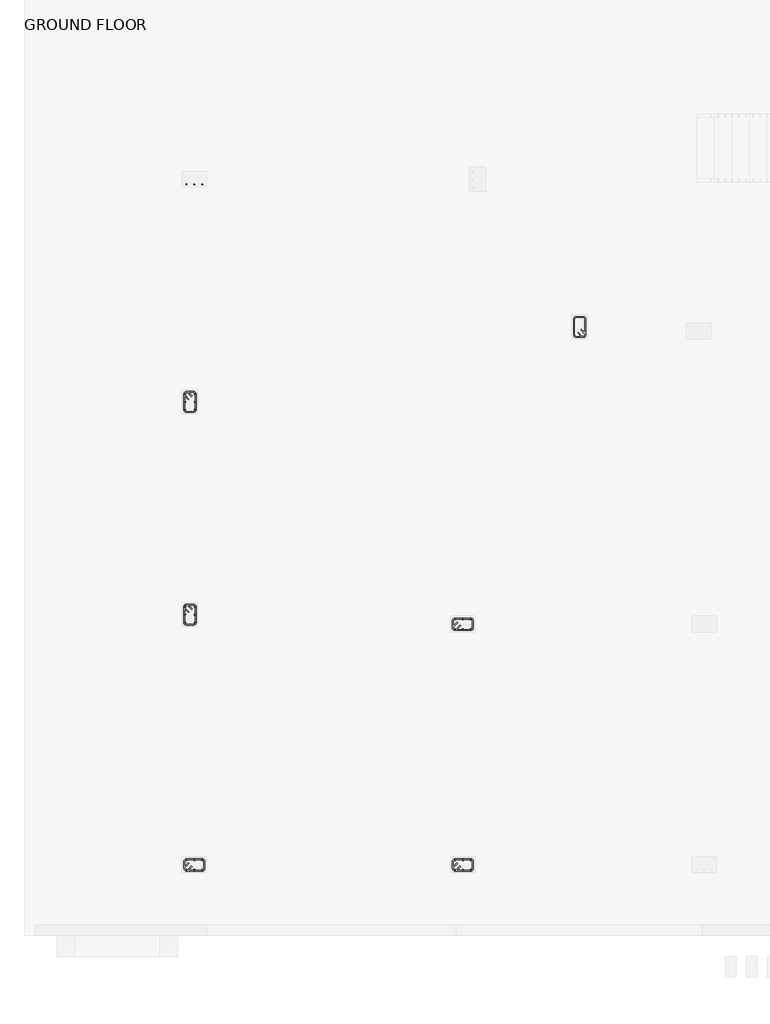
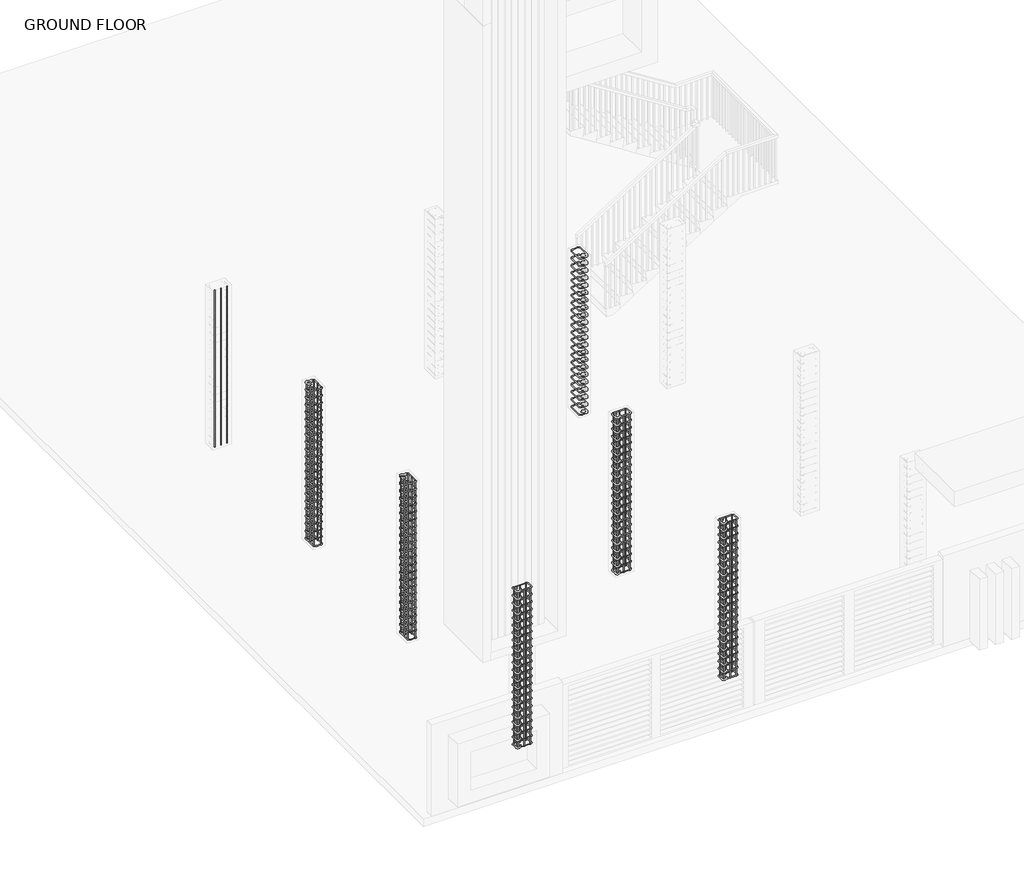
# One storey, part 3 of 7: 17 reinforcing bars.
"""IFC4 building model written with IfcOpenShell, lengths in millimetres."""

from ifc_helpers import new_model, si_unit, point, frame, origin, place, context, project, spatial, polyline, circle_curve, trimmed, segment, composite_curve, source, transform, mapped, element, save
from ifc_brep_helpers import swept_disk

model = new_model("IFC4")

# Units and contexts
model_context = context("Model", 3, world=origin())
ifc_project = project(units=[si_unit("LENGTHUNIT", "METRE", prefix="MILLI")], contexts=[model_context])

# Site, building, storey
site = spatial("IfcSite", under=ifc_project)
building = spatial("IfcBuilding", under=site)
storey = spatial("IfcBuildingStorey", under=building, Name="GROUND FLOOR", Elevation=0.0)

# Reinforcing bars
placement = place(None, origin())
reinforcing_bar_shape = source(origin(), model_context, "Body", "SolidModel", [
    swept_disk(composite_curve([segment(polyline([(-5960.0833787, -22.290066, 3175.0), (-5960.0833787, -22.290066, 25.4)]), True, "CONTINUOUS")], self_intersect=False), 6.35),
])
element("IfcReinforcingBar", 1, at=placement, inside=storey, context=model_context, shape_type="MappedRepresentation", body=[
    mapped(reinforcing_bar_shape, transform((0.0, 0.0, 0.0), x_axis=(1.0, 0.0, 0.0), y_axis=(0.0, 1.0, 0.0), z_axis=(0.0, 0.0, 1.0))),
    mapped(reinforcing_bar_shape, transform((-114.3, 0.0, 0.0), x_axis=(1.0, 0.0, 0.0), y_axis=(0.0, 1.0, 0.0), z_axis=(0.0, 0.0, 1.0))),
    mapped(reinforcing_bar_shape, transform((-228.6, 0.0, 0.0), x_axis=(1.0, 0.0, 0.0), y_axis=(0.0, 1.0, 0.0), z_axis=(0.0, 0.0, 1.0))),
])
reinforcing_bar_2_shape = source(origin(), model_context, "Body", "SolidModel", [
    swept_disk(composite_curve([segment(polyline([(-441.6142752, -2136.7078889, 3168.65), (-387.7327384, -2190.5894257, 3168.65)]), True, "CONTINUOUS"), segment(trimmed(circle_curve(frame((-410.1833787, -2213.040066, 3168.65), z_axis=(0.0, 0.0, -1.0), x_axis=(22.450640299999975, 22.450640300000032, 0.0)), 31.75), [point((-387.7327384, -2190.5894257, 3168.65))], [point((-410.1833787, -2244.790066, 3168.65))], True, "CARTESIAN"), True, "CONTINUOUS"), segment(polyline([(-410.1833787, -2244.790066, 3168.65), (-511.7833787, -2244.790066, 3168.65)]), True, "CONTINUOUS"), segment(trimmed(circle_curve(frame((-511.7833787, -2213.040066, 3168.65), z_axis=(0.0, 0.0, -1.0), x_axis=(0.0, -31.75, 0.0)), 31.75), [point((-511.7833787, -2244.790066, 3168.65))], [point((-543.5333787, -2213.040066, 3168.65))], True, "CARTESIAN"), True, "CONTINUOUS"), segment(polyline([(-543.5333787, -2213.040066, 3168.65), (-543.5333787, -1984.440066, 3168.65)]), True, "CONTINUOUS"), segment(trimmed(circle_curve(frame((-511.8768988, -1984.440066, 3171.0851138), z_axis=(0.07669649888473773, 0.0, -0.9970544855015816), x_axis=(-31.656479899999965, 0.0, -2.4351137999997263)), 31.75), [point((-543.5333787, -1984.440066, 3168.65))], [point((-511.8768988, -1952.690066, 3171.0851138))], True, "CARTESIAN"), True, "CONTINUOUS"), segment(polyline([(-511.8768988, -1952.690066, 3171.0851138), (-410.0898586, -1952.690066, 3178.9148862)]), True, "CONTINUOUS"), segment(trimmed(circle_curve(frame((-410.0898586, -1984.440066, 3178.9148862), z_axis=(0.07669649888473773, 0.0, -0.9970544855015816), x_axis=(0.0, 31.75, 0.0)), 31.75), [point((-410.0898586, -1952.690066, 3178.9148862))], [point((-378.4333787, -1984.440066, 3181.35))], True, "CARTESIAN"), True, "CONTINUOUS"), segment(polyline([(-378.4333787, -1984.440066, 3181.35), (-378.4333787, -2213.040066, 3181.35)]), True, "CONTINUOUS"), segment(trimmed(circle_curve(frame((-410.1833787, -2213.040066, 3181.35), z_axis=(0.0, 0.0, -1.0), x_axis=(31.75, 0.0, 0.0)), 31.75), [point((-378.4333787, -2213.040066, 3181.35))], [point((-432.634019, -2235.4907063, 3181.35))], True, "CARTESIAN"), True, "CONTINUOUS"), segment(polyline([(-432.634019, -2235.4907063, 3181.35), (-486.5155558, -2181.6091695, 3181.35)]), True, "CONTINUOUS")], self_intersect=False), 6.35),
])
element("IfcReinforcingBar", 2, at=placement, inside=storey, context=model_context, shape_type="MappedRepresentation", body=[
    mapped(reinforcing_bar_2_shape, transform((0.0, 0.0, 0.0), x_axis=(1.0, 0.0, 0.0), y_axis=(0.0, 1.0, 0.0), z_axis=(0.0, 0.0, 1.0))),
    mapped(reinforcing_bar_2_shape, transform((0.0, 0.0, -149.3761905), x_axis=(1.0, 0.0, 0.0), y_axis=(0.0, 1.0, 0.0), z_axis=(0.0, 0.0, 1.0))),
    mapped(reinforcing_bar_2_shape, transform((0.0, 0.0, -298.752381), x_axis=(1.0, 0.0, 0.0), y_axis=(0.0, 1.0, 0.0), z_axis=(0.0, 0.0, 1.0))),
    mapped(reinforcing_bar_2_shape, transform((0.0, 0.0, -448.1285714), x_axis=(1.0, 0.0, 0.0), y_axis=(0.0, 1.0, 0.0), z_axis=(0.0, 0.0, 1.0))),
    mapped(reinforcing_bar_2_shape, transform((0.0, 0.0, -597.5047619), x_axis=(1.0, 0.0, 0.0), y_axis=(0.0, 1.0, 0.0), z_axis=(0.0, 0.0, 1.0))),
    mapped(reinforcing_bar_2_shape, transform((0.0, 0.0, -746.8809524), x_axis=(1.0, 0.0, 0.0), y_axis=(0.0, 1.0, 0.0), z_axis=(0.0, 0.0, 1.0))),
    mapped(reinforcing_bar_2_shape, transform((0.0, 0.0, -896.2571429), x_axis=(1.0, 0.0, 0.0), y_axis=(0.0, 1.0, 0.0), z_axis=(0.0, 0.0, 1.0))),
    mapped(reinforcing_bar_2_shape, transform((0.0, 0.0, -1045.6333333), x_axis=(1.0, 0.0, 0.0), y_axis=(0.0, 1.0, 0.0), z_axis=(0.0, 0.0, 1.0))),
    mapped(reinforcing_bar_2_shape, transform((0.0, 0.0, -1195.0095238), x_axis=(1.0, 0.0, 0.0), y_axis=(0.0, 1.0, 0.0), z_axis=(0.0, 0.0, 1.0))),
    mapped(reinforcing_bar_2_shape, transform((0.0, 0.0, -1344.3857143), x_axis=(1.0, 0.0, 0.0), y_axis=(0.0, 1.0, 0.0), z_axis=(0.0, 0.0, 1.0))),
    mapped(reinforcing_bar_2_shape, transform((0.0, 0.0, -1493.7619048), x_axis=(1.0, 0.0, 0.0), y_axis=(0.0, 1.0, 0.0), z_axis=(0.0, 0.0, 1.0))),
    mapped(reinforcing_bar_2_shape, transform((0.0, 0.0, -1643.1380952), x_axis=(1.0, 0.0, 0.0), y_axis=(0.0, 1.0, 0.0), z_axis=(0.0, 0.0, 1.0))),
    mapped(reinforcing_bar_2_shape, transform((0.0, 0.0, -1792.5142857), x_axis=(1.0, 0.0, 0.0), y_axis=(0.0, 1.0, 0.0), z_axis=(0.0, 0.0, 1.0))),
    mapped(reinforcing_bar_2_shape, transform((0.0, 0.0, -1941.8904762), x_axis=(1.0, 0.0, 0.0), y_axis=(0.0, 1.0, 0.0), z_axis=(0.0, 0.0, 1.0))),
    mapped(reinforcing_bar_2_shape, transform((0.0, 0.0, -2091.2666667), x_axis=(1.0, 0.0, 0.0), y_axis=(0.0, 1.0, 0.0), z_axis=(0.0, 0.0, 1.0))),
    mapped(reinforcing_bar_2_shape, transform((0.0, 0.0, -2240.6428571), x_axis=(1.0, 0.0, 0.0), y_axis=(0.0, 1.0, 0.0), z_axis=(0.0, 0.0, 1.0))),
    mapped(reinforcing_bar_2_shape, transform((0.0, 0.0, -2390.0190476), x_axis=(1.0, 0.0, 0.0), y_axis=(0.0, 1.0, 0.0), z_axis=(0.0, 0.0, 1.0))),
    mapped(reinforcing_bar_2_shape, transform((0.0, 0.0, -2539.3952381), x_axis=(1.0, 0.0, 0.0), y_axis=(0.0, 1.0, 0.0), z_axis=(0.0, 0.0, 1.0))),
    mapped(reinforcing_bar_2_shape, transform((0.0, 0.0, -2688.7714286), x_axis=(1.0, 0.0, 0.0), y_axis=(0.0, 1.0, 0.0), z_axis=(0.0, 0.0, 1.0))),
    mapped(reinforcing_bar_2_shape, transform((0.0, 0.0, -2838.147619), x_axis=(1.0, 0.0, 0.0), y_axis=(0.0, 1.0, 0.0), z_axis=(0.0, 0.0, 1.0))),
    mapped(reinforcing_bar_2_shape, transform((0.0, 0.0, -2987.5238095), x_axis=(1.0, 0.0, 0.0), y_axis=(0.0, 1.0, 0.0), z_axis=(0.0, 0.0, 1.0))),
    mapped(reinforcing_bar_2_shape, transform((0.0, 0.0, -3136.9), x_axis=(1.0, 0.0, 0.0), y_axis=(0.0, 1.0, 0.0), z_axis=(0.0, 0.0, 1.0))),
])
reinforcing_bar_3_shape = source(origin(), model_context, "Body", "SolidModel", [
    swept_disk(composite_curve([segment(polyline([(-2200.7512017, -6448.8091695, 3168.65), (-2254.6327384, -6502.6907063, 3168.65)]), True, "CONTINUOUS"), segment(trimmed(circle_curve(frame((-2277.0833787, -6480.240066, 3168.65), z_axis=(0.0, 0.0, -1.0), x_axis=(22.450640300000032, -22.450640299999577, 0.0)), 31.75), [point((-2254.6327384, -6502.6907063, 3168.65))], [point((-2308.8333787, -6480.240066, 3168.65))], True, "CARTESIAN"), True, "CONTINUOUS"), segment(polyline([(-2308.8333787, -6480.240066, 3168.65), (-2308.8333787, -6378.640066, 3168.65)]), True, "CONTINUOUS"), segment(trimmed(circle_curve(frame((-2277.0833787, -6378.640066, 3168.65), z_axis=(0.0, 0.0, -1.0), x_axis=(-31.75, 0.0, 0.0)), 31.75), [point((-2308.8333787, -6378.640066, 3168.65))], [point((-2277.0833787, -6346.890066, 3168.65))], True, "CARTESIAN"), True, "CONTINUOUS"), segment(polyline([(-2277.0833787, -6346.890066, 3168.65), (-2048.4833787, -6346.890066, 3168.65)]), True, "CONTINUOUS"), segment(trimmed(circle_curve(frame((-2048.4833787, -6378.5465459, 3171.0851138), z_axis=(0.0, -0.07669649888473773, -0.9970544855015816), x_axis=(0.0, 31.656479899999795, -2.4351137999997263)), 31.75), [point((-2048.4833787, -6346.890066, 3168.65))], [point((-2016.7333787, -6378.5465459, 3171.0851138))], True, "CARTESIAN"), True, "CONTINUOUS"), segment(polyline([(-2016.7333787, -6378.5465459, 3171.0851138), (-2016.7333787, -6480.3335861, 3178.9148862)]), True, "CONTINUOUS"), segment(trimmed(circle_curve(frame((-2048.4833787, -6480.3335861, 3178.9148862), z_axis=(0.0, -0.07669649888473773, -0.9970544855015816), x_axis=(31.749999999999773, 0.0, 0.0)), 31.75), [point((-2016.7333787, -6480.3335861, 3178.9148862))], [point((-2048.4833787, -6511.990066, 3181.35))], True, "CARTESIAN"), True, "CONTINUOUS"), segment(polyline([(-2048.4833787, -6511.990066, 3181.35), (-2277.0833787, -6511.990066, 3181.35)]), True, "CONTINUOUS"), segment(trimmed(circle_curve(frame((-2277.0833787, -6480.240066, 3181.35), z_axis=(0.0, 0.0, -1.0), x_axis=(0.0, -31.75, 0.0)), 31.75), [point((-2277.0833787, -6511.990066, 3181.35))], [point((-2299.534019, -6457.7894257, 3181.35))], True, "CARTESIAN"), True, "CONTINUOUS"), segment(polyline([(-2299.534019, -6457.7894257, 3181.35), (-2245.6524823, -6403.9078889, 3181.35)]), True, "CONTINUOUS")], self_intersect=False), 6.35),
])
element("IfcReinforcingBar", 3, at=placement, inside=storey, context=model_context, shape_type="MappedRepresentation", body=[
    mapped(reinforcing_bar_3_shape, transform((0.0, 0.0, 0.0), x_axis=(1.0, 0.0, 0.0), y_axis=(0.0, 1.0, 0.0), z_axis=(0.0, 0.0, 1.0))),
    mapped(reinforcing_bar_3_shape, transform((0.0, 0.0, -149.3761905), x_axis=(1.0, 0.0, 0.0), y_axis=(0.0, 1.0, 0.0), z_axis=(0.0, 0.0, 1.0))),
    mapped(reinforcing_bar_3_shape, transform((0.0, 0.0, -298.752381), x_axis=(1.0, 0.0, 0.0), y_axis=(0.0, 1.0, 0.0), z_axis=(0.0, 0.0, 1.0))),
    mapped(reinforcing_bar_3_shape, transform((0.0, 0.0, -448.1285714), x_axis=(1.0, 0.0, 0.0), y_axis=(0.0, 1.0, 0.0), z_axis=(0.0, 0.0, 1.0))),
    mapped(reinforcing_bar_3_shape, transform((0.0, 0.0, -597.5047619), x_axis=(1.0, 0.0, 0.0), y_axis=(0.0, 1.0, 0.0), z_axis=(0.0, 0.0, 1.0))),
    mapped(reinforcing_bar_3_shape, transform((0.0, 0.0, -746.8809524), x_axis=(1.0, 0.0, 0.0), y_axis=(0.0, 1.0, 0.0), z_axis=(0.0, 0.0, 1.0))),
    mapped(reinforcing_bar_3_shape, transform((0.0, 0.0, -896.2571429), x_axis=(1.0, 0.0, 0.0), y_axis=(0.0, 1.0, 0.0), z_axis=(0.0, 0.0, 1.0))),
    mapped(reinforcing_bar_3_shape, transform((0.0, 0.0, -1045.6333333), x_axis=(1.0, 0.0, 0.0), y_axis=(0.0, 1.0, 0.0), z_axis=(0.0, 0.0, 1.0))),
    mapped(reinforcing_bar_3_shape, transform((0.0, 0.0, -1195.0095238), x_axis=(1.0, 0.0, 0.0), y_axis=(0.0, 1.0, 0.0), z_axis=(0.0, 0.0, 1.0))),
    mapped(reinforcing_bar_3_shape, transform((0.0, 0.0, -1344.3857143), x_axis=(1.0, 0.0, 0.0), y_axis=(0.0, 1.0, 0.0), z_axis=(0.0, 0.0, 1.0))),
    mapped(reinforcing_bar_3_shape, transform((0.0, 0.0, -1493.7619048), x_axis=(1.0, 0.0, 0.0), y_axis=(0.0, 1.0, 0.0), z_axis=(0.0, 0.0, 1.0))),
    mapped(reinforcing_bar_3_shape, transform((0.0, 0.0, -1643.1380952), x_axis=(1.0, 0.0, 0.0), y_axis=(0.0, 1.0, 0.0), z_axis=(0.0, 0.0, 1.0))),
    mapped(reinforcing_bar_3_shape, transform((0.0, 0.0, -1792.5142857), x_axis=(1.0, 0.0, 0.0), y_axis=(0.0, 1.0, 0.0), z_axis=(0.0, 0.0, 1.0))),
    mapped(reinforcing_bar_3_shape, transform((0.0, 0.0, -1941.8904762), x_axis=(1.0, 0.0, 0.0), y_axis=(0.0, 1.0, 0.0), z_axis=(0.0, 0.0, 1.0))),
    mapped(reinforcing_bar_3_shape, transform((0.0, 0.0, -2091.2666667), x_axis=(1.0, 0.0, 0.0), y_axis=(0.0, 1.0, 0.0), z_axis=(0.0, 0.0, 1.0))),
    mapped(reinforcing_bar_3_shape, transform((0.0, 0.0, -2240.6428571), x_axis=(1.0, 0.0, 0.0), y_axis=(0.0, 1.0, 0.0), z_axis=(0.0, 0.0, 1.0))),
    mapped(reinforcing_bar_3_shape, transform((0.0, 0.0, -2390.0190476), x_axis=(1.0, 0.0, 0.0), y_axis=(0.0, 1.0, 0.0), z_axis=(0.0, 0.0, 1.0))),
    mapped(reinforcing_bar_3_shape, transform((0.0, 0.0, -2539.3952381), x_axis=(1.0, 0.0, 0.0), y_axis=(0.0, 1.0, 0.0), z_axis=(0.0, 0.0, 1.0))),
    mapped(reinforcing_bar_3_shape, transform((0.0, 0.0, -2688.7714286), x_axis=(1.0, 0.0, 0.0), y_axis=(0.0, 1.0, 0.0), z_axis=(0.0, 0.0, 1.0))),
    mapped(reinforcing_bar_3_shape, transform((0.0, 0.0, -2838.147619), x_axis=(1.0, 0.0, 0.0), y_axis=(0.0, 1.0, 0.0), z_axis=(0.0, 0.0, 1.0))),
    mapped(reinforcing_bar_3_shape, transform((0.0, 0.0, -2987.5238095), x_axis=(1.0, 0.0, 0.0), y_axis=(0.0, 1.0, 0.0), z_axis=(0.0, 0.0, 1.0))),
    mapped(reinforcing_bar_3_shape, transform((0.0, 0.0, -3136.9), x_axis=(1.0, 0.0, 0.0), y_axis=(0.0, 1.0, 0.0), z_axis=(0.0, 0.0, 1.0))),
])
reinforcing_bar_4_shape = source(origin(), model_context, "Body", "SolidModel", [
    swept_disk(composite_curve([segment(polyline([(-2277.0833787, -6359.590066, 3175.0), (-2277.0833787, -6359.590066, 25.4)]), True, "CONTINUOUS")], self_intersect=False), 6.35),
])
element("IfcReinforcingBar", 4, at=placement, inside=storey, context=model_context, shape_type="MappedRepresentation", body=[
    mapped(reinforcing_bar_4_shape, transform((0.0, 0.0, 0.0), x_axis=(1.0, 0.0, 0.0), y_axis=(0.0, 1.0, 0.0), z_axis=(0.0, 0.0, 1.0))),
    mapped(reinforcing_bar_4_shape, transform((114.3, 0.0, 0.0), x_axis=(1.0, 0.0, 0.0), y_axis=(0.0, 1.0, 0.0), z_axis=(0.0, 0.0, 1.0))),
    mapped(reinforcing_bar_4_shape, transform((228.6, 0.0, 0.0), x_axis=(1.0, 0.0, 0.0), y_axis=(0.0, 1.0, 0.0), z_axis=(0.0, 0.0, 1.0))),
])
reinforcing_bar_5_shape = source(origin(), model_context, "Body", "SolidModel", [
    swept_disk(composite_curve([segment(polyline([(-2277.0833787, -6499.290066, 25.4), (-2277.0833787, -6499.290066, 3175.0)]), True, "CONTINUOUS")], self_intersect=False), 6.35),
])
element("IfcReinforcingBar", 5, at=placement, inside=storey, context=model_context, shape_type="MappedRepresentation", body=[
    mapped(reinforcing_bar_5_shape, transform((0.0, 0.0, 0.0), x_axis=(1.0, 0.0, 0.0), y_axis=(0.0, 1.0, 0.0), z_axis=(0.0, 0.0, 1.0))),
    mapped(reinforcing_bar_5_shape, transform((114.3, 0.0, 0.0), x_axis=(1.0, 0.0, 0.0), y_axis=(0.0, 1.0, 0.0), z_axis=(0.0, 0.0, 1.0))),
    mapped(reinforcing_bar_5_shape, transform((228.6, 0.0, 0.0), x_axis=(1.0, 0.0, 0.0), y_axis=(0.0, 1.0, 0.0), z_axis=(0.0, 0.0, 1.0))),
])
reinforcing_bar_6_shape = source(origin(), model_context, "Body", "SolidModel", [
    swept_disk(composite_curve([segment(polyline([(-6157.2524823, -3152.972243, 3168.65), (-6211.134019, -3099.0907063, 3168.65)]), True, "CONTINUOUS"), segment(trimmed(circle_curve(frame((-6188.6833787, -3076.640066, 3168.65), z_axis=(0.0, 0.0, -1.0), x_axis=(-22.450640300000487, -22.450640300000032, 0.0)), 31.75), [point((-6211.134019, -3099.0907063, 3168.65))], [point((-6188.6833787, -3044.890066, 3168.65))], True, "CARTESIAN"), True, "CONTINUOUS"), segment(polyline([(-6188.6833787, -3044.890066, 3168.65), (-6087.0833787, -3044.890066, 3168.65)]), True, "CONTINUOUS"), segment(trimmed(circle_curve(frame((-6087.0833787, -3076.640066, 3168.65), z_axis=(0.0, 0.0, -1.0), x_axis=(0.0, 31.75, 0.0)), 31.75), [point((-6087.0833787, -3044.890066, 3168.65))], [point((-6055.3333787, -3076.640066, 3168.65))], True, "CARTESIAN"), True, "CONTINUOUS"), segment(polyline([(-6055.3333787, -3076.640066, 3168.65), (-6055.3333787, -3305.240066, 3168.65)]), True, "CONTINUOUS"), segment(trimmed(circle_curve(frame((-6086.9898586, -3305.240066, 3171.0851138), z_axis=(-0.07669649888473773, 0.0, -0.9970544855015816), x_axis=(31.656479899999795, 0.0, -2.4351137999997263)), 31.75), [point((-6055.3333787, -3305.240066, 3168.65))], [point((-6086.9898586, -3336.990066, 3171.0851138))], True, "CARTESIAN"), True, "CONTINUOUS"), segment(polyline([(-6086.9898586, -3336.990066, 3171.0851138), (-6188.7768988, -3336.990066, 3178.9148862)]), True, "CONTINUOUS"), segment(trimmed(circle_curve(frame((-6188.7768988, -3305.240066, 3178.9148862), z_axis=(-0.07669649888473773, 0.0, -0.9970544855015816), x_axis=(0.0, -31.75, 0.0)), 31.75), [point((-6188.7768988, -3336.990066, 3178.9148862))], [point((-6220.4333787, -3305.240066, 3181.35))], True, "CARTESIAN"), True, "CONTINUOUS"), segment(polyline([(-6220.4333787, -3305.240066, 3181.35), (-6220.4333787, -3076.640066, 3181.35)]), True, "CONTINUOUS"), segment(trimmed(circle_curve(frame((-6188.6833787, -3076.640066, 3181.35), z_axis=(0.0, 0.0, -1.0), x_axis=(-31.75, 0.0, 0.0)), 31.75), [point((-6220.4333787, -3076.640066, 3181.35))], [point((-6166.2327384, -3054.1894257, 3181.35))], True, "CARTESIAN"), True, "CONTINUOUS"), segment(polyline([(-6166.2327384, -3054.1894257, 3181.35), (-6112.3512017, -3108.0709624, 3181.35)]), True, "CONTINUOUS")], self_intersect=False), 6.35),
])
element("IfcReinforcingBar", 6, at=placement, inside=storey, context=model_context, shape_type="MappedRepresentation", body=[
    mapped(reinforcing_bar_6_shape, transform((0.0, 0.0, 0.0), x_axis=(1.0, 0.0, 0.0), y_axis=(0.0, 1.0, 0.0), z_axis=(0.0, 0.0, 1.0))),
    mapped(reinforcing_bar_6_shape, transform((0.0, 0.0, -149.3761905), x_axis=(1.0, 0.0, 0.0), y_axis=(0.0, 1.0, 0.0), z_axis=(0.0, 0.0, 1.0))),
    mapped(reinforcing_bar_6_shape, transform((0.0, 0.0, -298.752381), x_axis=(1.0, 0.0, 0.0), y_axis=(0.0, 1.0, 0.0), z_axis=(0.0, 0.0, 1.0))),
    mapped(reinforcing_bar_6_shape, transform((0.0, 0.0, -448.1285714), x_axis=(1.0, 0.0, 0.0), y_axis=(0.0, 1.0, 0.0), z_axis=(0.0, 0.0, 1.0))),
    mapped(reinforcing_bar_6_shape, transform((0.0, 0.0, -597.5047619), x_axis=(1.0, 0.0, 0.0), y_axis=(0.0, 1.0, 0.0), z_axis=(0.0, 0.0, 1.0))),
    mapped(reinforcing_bar_6_shape, transform((0.0, 0.0, -746.8809524), x_axis=(1.0, 0.0, 0.0), y_axis=(0.0, 1.0, 0.0), z_axis=(0.0, 0.0, 1.0))),
    mapped(reinforcing_bar_6_shape, transform((0.0, 0.0, -896.2571429), x_axis=(1.0, 0.0, 0.0), y_axis=(0.0, 1.0, 0.0), z_axis=(0.0, 0.0, 1.0))),
    mapped(reinforcing_bar_6_shape, transform((0.0, 0.0, -1045.6333333), x_axis=(1.0, 0.0, 0.0), y_axis=(0.0, 1.0, 0.0), z_axis=(0.0, 0.0, 1.0))),
    mapped(reinforcing_bar_6_shape, transform((0.0, 0.0, -1195.0095238), x_axis=(1.0, 0.0, 0.0), y_axis=(0.0, 1.0, 0.0), z_axis=(0.0, 0.0, 1.0))),
    mapped(reinforcing_bar_6_shape, transform((0.0, 0.0, -1344.3857143), x_axis=(1.0, 0.0, 0.0), y_axis=(0.0, 1.0, 0.0), z_axis=(0.0, 0.0, 1.0))),
    mapped(reinforcing_bar_6_shape, transform((0.0, 0.0, -1493.7619048), x_axis=(1.0, 0.0, 0.0), y_axis=(0.0, 1.0, 0.0), z_axis=(0.0, 0.0, 1.0))),
    mapped(reinforcing_bar_6_shape, transform((0.0, 0.0, -1643.1380952), x_axis=(1.0, 0.0, 0.0), y_axis=(0.0, 1.0, 0.0), z_axis=(0.0, 0.0, 1.0))),
    mapped(reinforcing_bar_6_shape, transform((0.0, 0.0, -1792.5142857), x_axis=(1.0, 0.0, 0.0), y_axis=(0.0, 1.0, 0.0), z_axis=(0.0, 0.0, 1.0))),
    mapped(reinforcing_bar_6_shape, transform((0.0, 0.0, -1941.8904762), x_axis=(1.0, 0.0, 0.0), y_axis=(0.0, 1.0, 0.0), z_axis=(0.0, 0.0, 1.0))),
    mapped(reinforcing_bar_6_shape, transform((0.0, 0.0, -2091.2666667), x_axis=(1.0, 0.0, 0.0), y_axis=(0.0, 1.0, 0.0), z_axis=(0.0, 0.0, 1.0))),
    mapped(reinforcing_bar_6_shape, transform((0.0, 0.0, -2240.6428571), x_axis=(1.0, 0.0, 0.0), y_axis=(0.0, 1.0, 0.0), z_axis=(0.0, 0.0, 1.0))),
    mapped(reinforcing_bar_6_shape, transform((0.0, 0.0, -2390.0190476), x_axis=(1.0, 0.0, 0.0), y_axis=(0.0, 1.0, 0.0), z_axis=(0.0, 0.0, 1.0))),
    mapped(reinforcing_bar_6_shape, transform((0.0, 0.0, -2539.3952381), x_axis=(1.0, 0.0, 0.0), y_axis=(0.0, 1.0, 0.0), z_axis=(0.0, 0.0, 1.0))),
    mapped(reinforcing_bar_6_shape, transform((0.0, 0.0, -2688.7714286), x_axis=(1.0, 0.0, 0.0), y_axis=(0.0, 1.0, 0.0), z_axis=(0.0, 0.0, 1.0))),
    mapped(reinforcing_bar_6_shape, transform((0.0, 0.0, -2838.147619), x_axis=(1.0, 0.0, 0.0), y_axis=(0.0, 1.0, 0.0), z_axis=(0.0, 0.0, 1.0))),
    mapped(reinforcing_bar_6_shape, transform((0.0, 0.0, -2987.5238095), x_axis=(1.0, 0.0, 0.0), y_axis=(0.0, 1.0, 0.0), z_axis=(0.0, 0.0, 1.0))),
    mapped(reinforcing_bar_6_shape, transform((0.0, 0.0, -3136.9), x_axis=(1.0, 0.0, 0.0), y_axis=(0.0, 1.0, 0.0), z_axis=(0.0, 0.0, 1.0))),
])
reinforcing_bar_7_shape = source(origin(), model_context, "Body", "SolidModel", [
    swept_disk(composite_curve([segment(polyline([(-6068.0333787, -3076.640066, 3175.0), (-6068.0333787, -3076.640066, 25.4)]), True, "CONTINUOUS")], self_intersect=False), 6.35),
])
element("IfcReinforcingBar", 7, at=placement, inside=storey, context=model_context, shape_type="MappedRepresentation", body=[
    mapped(reinforcing_bar_7_shape, transform((0.0, 0.0, 0.0), x_axis=(1.0, 0.0, 0.0), y_axis=(0.0, 1.0, 0.0), z_axis=(0.0, 0.0, 1.0))),
    mapped(reinforcing_bar_7_shape, transform((0.0, -114.3, 0.0), x_axis=(1.0, 0.0, 0.0), y_axis=(0.0, 1.0, 0.0), z_axis=(0.0, 0.0, 1.0))),
    mapped(reinforcing_bar_7_shape, transform((0.0, -228.6, 0.0), x_axis=(1.0, 0.0, 0.0), y_axis=(0.0, 1.0, 0.0), z_axis=(0.0, 0.0, 1.0))),
])
reinforcing_bar_8_shape = source(origin(), model_context, "Body", "SolidModel", [
    swept_disk(composite_curve([segment(polyline([(-6207.7333787, -3076.640066, 25.4), (-6207.7333787, -3076.640066, 3175.0)]), True, "CONTINUOUS")], self_intersect=False), 6.35),
])
element("IfcReinforcingBar", 8, at=placement, inside=storey, context=model_context, shape_type="MappedRepresentation", body=[
    mapped(reinforcing_bar_8_shape, transform((0.0, 0.0, 0.0), x_axis=(1.0, 0.0, 0.0), y_axis=(0.0, 1.0, 0.0), z_axis=(0.0, 0.0, 1.0))),
    mapped(reinforcing_bar_8_shape, transform((0.0, -114.3, 0.0), x_axis=(1.0, 0.0, 0.0), y_axis=(0.0, 1.0, 0.0), z_axis=(0.0, 0.0, 1.0))),
    mapped(reinforcing_bar_8_shape, transform((0.0, -228.6, 0.0), x_axis=(1.0, 0.0, 0.0), y_axis=(0.0, 1.0, 0.0), z_axis=(0.0, 0.0, 1.0))),
])
reinforcing_bar_9_shape = source(origin(), model_context, "Body", "SolidModel", [
    swept_disk(composite_curve([segment(polyline([(-2200.7512017, -9954.0091695, 3168.65), (-2254.6327384, -10007.8907063, 3168.65)]), True, "CONTINUOUS"), segment(trimmed(circle_curve(frame((-2277.0833787, -9985.440066, 3168.65), z_axis=(0.0, 0.0, -1.0), x_axis=(22.450640300000032, -22.450640300001396, 0.0)), 31.75), [point((-2254.6327384, -10007.8907063, 3168.65))], [point((-2308.8333787, -9985.440066, 3168.65))], True, "CARTESIAN"), True, "CONTINUOUS"), segment(polyline([(-2308.8333787, -9985.440066, 3168.65), (-2308.8333787, -9883.840066, 3168.65)]), True, "CONTINUOUS"), segment(trimmed(circle_curve(frame((-2277.0833787, -9883.840066, 3168.65), z_axis=(0.0, 0.0, -1.0), x_axis=(-31.75, 0.0, 0.0)), 31.75), [point((-2308.8333787, -9883.840066, 3168.65))], [point((-2277.0833787, -9852.090066, 3168.65))], True, "CARTESIAN"), True, "CONTINUOUS"), segment(polyline([(-2277.0833787, -9852.090066, 3168.65), (-2048.4833787, -9852.090066, 3168.65)]), True, "CONTINUOUS"), segment(trimmed(circle_curve(frame((-2048.4833787, -9883.7465459, 3171.0851138), z_axis=(0.0, -0.07669649888473773, -0.9970544855015816), x_axis=(0.0, 31.656479899998885, -2.4351137999997263)), 31.75), [point((-2048.4833787, -9852.090066, 3168.65))], [point((-2016.7333787, -9883.7465459, 3171.0851138))], True, "CARTESIAN"), True, "CONTINUOUS"), segment(polyline([(-2016.7333787, -9883.7465459, 3171.0851138), (-2016.7333787, -9985.5335861, 3178.9148862)]), True, "CONTINUOUS"), segment(trimmed(circle_curve(frame((-2048.4833787, -9985.5335861, 3178.9148862), z_axis=(0.0, -0.07669649888473773, -0.9970544855015816), x_axis=(31.749999999999773, 0.0, 0.0)), 31.75), [point((-2016.7333787, -9985.5335861, 3178.9148862))], [point((-2048.4833787, -10017.190066, 3181.35))], True, "CARTESIAN"), True, "CONTINUOUS"), segment(polyline([(-2048.4833787, -10017.190066, 3181.35), (-2277.0833787, -10017.190066, 3181.35)]), True, "CONTINUOUS"), segment(trimmed(circle_curve(frame((-2277.0833787, -9985.440066, 3181.35), z_axis=(0.0, 0.0, -1.0), x_axis=(0.0, -31.75, 0.0)), 31.75), [point((-2277.0833787, -10017.190066, 3181.35))], [point((-2299.534019, -9962.9894257, 3181.35))], True, "CARTESIAN"), True, "CONTINUOUS"), segment(polyline([(-2299.534019, -9962.9894257, 3181.35), (-2245.6524823, -9909.1078889, 3181.35)]), True, "CONTINUOUS")], self_intersect=False), 6.35),
])
element("IfcReinforcingBar", 9, at=placement, inside=storey, context=model_context, shape_type="MappedRepresentation", body=[
    mapped(reinforcing_bar_9_shape, transform((0.0, 0.0, 0.0), x_axis=(1.0, 0.0, 0.0), y_axis=(0.0, 1.0, 0.0), z_axis=(0.0, 0.0, 1.0))),
    mapped(reinforcing_bar_9_shape, transform((0.0, 0.0, -149.3761905), x_axis=(1.0, 0.0, 0.0), y_axis=(0.0, 1.0, 0.0), z_axis=(0.0, 0.0, 1.0))),
    mapped(reinforcing_bar_9_shape, transform((0.0, 0.0, -298.752381), x_axis=(1.0, 0.0, 0.0), y_axis=(0.0, 1.0, 0.0), z_axis=(0.0, 0.0, 1.0))),
    mapped(reinforcing_bar_9_shape, transform((0.0, 0.0, -448.1285714), x_axis=(1.0, 0.0, 0.0), y_axis=(0.0, 1.0, 0.0), z_axis=(0.0, 0.0, 1.0))),
    mapped(reinforcing_bar_9_shape, transform((0.0, 0.0, -597.5047619), x_axis=(1.0, 0.0, 0.0), y_axis=(0.0, 1.0, 0.0), z_axis=(0.0, 0.0, 1.0))),
    mapped(reinforcing_bar_9_shape, transform((0.0, 0.0, -746.8809524), x_axis=(1.0, 0.0, 0.0), y_axis=(0.0, 1.0, 0.0), z_axis=(0.0, 0.0, 1.0))),
    mapped(reinforcing_bar_9_shape, transform((0.0, 0.0, -896.2571429), x_axis=(1.0, 0.0, 0.0), y_axis=(0.0, 1.0, 0.0), z_axis=(0.0, 0.0, 1.0))),
    mapped(reinforcing_bar_9_shape, transform((0.0, 0.0, -1045.6333333), x_axis=(1.0, 0.0, 0.0), y_axis=(0.0, 1.0, 0.0), z_axis=(0.0, 0.0, 1.0))),
    mapped(reinforcing_bar_9_shape, transform((0.0, 0.0, -1195.0095238), x_axis=(1.0, 0.0, 0.0), y_axis=(0.0, 1.0, 0.0), z_axis=(0.0, 0.0, 1.0))),
    mapped(reinforcing_bar_9_shape, transform((0.0, 0.0, -1344.3857143), x_axis=(1.0, 0.0, 0.0), y_axis=(0.0, 1.0, 0.0), z_axis=(0.0, 0.0, 1.0))),
    mapped(reinforcing_bar_9_shape, transform((0.0, 0.0, -1493.7619048), x_axis=(1.0, 0.0, 0.0), y_axis=(0.0, 1.0, 0.0), z_axis=(0.0, 0.0, 1.0))),
    mapped(reinforcing_bar_9_shape, transform((0.0, 0.0, -1643.1380952), x_axis=(1.0, 0.0, 0.0), y_axis=(0.0, 1.0, 0.0), z_axis=(0.0, 0.0, 1.0))),
    mapped(reinforcing_bar_9_shape, transform((0.0, 0.0, -1792.5142857), x_axis=(1.0, 0.0, 0.0), y_axis=(0.0, 1.0, 0.0), z_axis=(0.0, 0.0, 1.0))),
    mapped(reinforcing_bar_9_shape, transform((0.0, 0.0, -1941.8904762), x_axis=(1.0, 0.0, 0.0), y_axis=(0.0, 1.0, 0.0), z_axis=(0.0, 0.0, 1.0))),
    mapped(reinforcing_bar_9_shape, transform((0.0, 0.0, -2091.2666667), x_axis=(1.0, 0.0, 0.0), y_axis=(0.0, 1.0, 0.0), z_axis=(0.0, 0.0, 1.0))),
    mapped(reinforcing_bar_9_shape, transform((0.0, 0.0, -2240.6428571), x_axis=(1.0, 0.0, 0.0), y_axis=(0.0, 1.0, 0.0), z_axis=(0.0, 0.0, 1.0))),
    mapped(reinforcing_bar_9_shape, transform((0.0, 0.0, -2390.0190476), x_axis=(1.0, 0.0, 0.0), y_axis=(0.0, 1.0, 0.0), z_axis=(0.0, 0.0, 1.0))),
    mapped(reinforcing_bar_9_shape, transform((0.0, 0.0, -2539.3952381), x_axis=(1.0, 0.0, 0.0), y_axis=(0.0, 1.0, 0.0), z_axis=(0.0, 0.0, 1.0))),
    mapped(reinforcing_bar_9_shape, transform((0.0, 0.0, -2688.7714286), x_axis=(1.0, 0.0, 0.0), y_axis=(0.0, 1.0, 0.0), z_axis=(0.0, 0.0, 1.0))),
    mapped(reinforcing_bar_9_shape, transform((0.0, 0.0, -2838.147619), x_axis=(1.0, 0.0, 0.0), y_axis=(0.0, 1.0, 0.0), z_axis=(0.0, 0.0, 1.0))),
    mapped(reinforcing_bar_9_shape, transform((0.0, 0.0, -2987.5238095), x_axis=(1.0, 0.0, 0.0), y_axis=(0.0, 1.0, 0.0), z_axis=(0.0, 0.0, 1.0))),
    mapped(reinforcing_bar_9_shape, transform((0.0, 0.0, -3136.9), x_axis=(1.0, 0.0, 0.0), y_axis=(0.0, 1.0, 0.0), z_axis=(0.0, 0.0, 1.0))),
])
reinforcing_bar_10_shape = source(origin(), model_context, "Body", "SolidModel", [
    swept_disk(composite_curve([segment(polyline([(-2277.0833787, -9864.790066, 3175.0), (-2277.0833787, -9864.790066, 25.4)]), True, "CONTINUOUS")], self_intersect=False), 6.35),
])
element("IfcReinforcingBar", 10, at=placement, inside=storey, context=model_context, shape_type="MappedRepresentation", body=[
    mapped(reinforcing_bar_10_shape, transform((0.0, 0.0, 0.0), x_axis=(1.0, 0.0, 0.0), y_axis=(0.0, 1.0, 0.0), z_axis=(0.0, 0.0, 1.0))),
    mapped(reinforcing_bar_10_shape, transform((114.3, 0.0, 0.0), x_axis=(1.0, 0.0, 0.0), y_axis=(0.0, 1.0, 0.0), z_axis=(0.0, 0.0, 1.0))),
    mapped(reinforcing_bar_10_shape, transform((228.6, 0.0, 0.0), x_axis=(1.0, 0.0, 0.0), y_axis=(0.0, 1.0, 0.0), z_axis=(0.0, 0.0, 1.0))),
])
reinforcing_bar_11_shape = source(origin(), model_context, "Body", "SolidModel", [
    swept_disk(composite_curve([segment(polyline([(-2277.0833787, -10004.490066, 25.4), (-2277.0833787, -10004.490066, 3175.0)]), True, "CONTINUOUS")], self_intersect=False), 6.35),
])
element("IfcReinforcingBar", 11, at=placement, inside=storey, context=model_context, shape_type="MappedRepresentation", body=[
    mapped(reinforcing_bar_11_shape, transform((0.0, 0.0, 0.0), x_axis=(1.0, 0.0, 0.0), y_axis=(0.0, 1.0, 0.0), z_axis=(0.0, 0.0, 1.0))),
    mapped(reinforcing_bar_11_shape, transform((114.3, 0.0, 0.0), x_axis=(1.0, 0.0, 0.0), y_axis=(0.0, 1.0, 0.0), z_axis=(0.0, 0.0, 1.0))),
    mapped(reinforcing_bar_11_shape, transform((228.6, 0.0, 0.0), x_axis=(1.0, 0.0, 0.0), y_axis=(0.0, 1.0, 0.0), z_axis=(0.0, 0.0, 1.0))),
])
reinforcing_bar_12_shape = source(origin(), model_context, "Body", "SolidModel", [
    swept_disk(composite_curve([segment(polyline([(-6112.3512017, -9954.0091695, 3168.65), (-6166.2327384, -10007.8907063, 3168.65)]), True, "CONTINUOUS"), segment(trimmed(circle_curve(frame((-6188.6833787, -9985.440066, 3168.65), z_axis=(0.0, 0.0, -1.0), x_axis=(22.450640299999577, -22.450640300001396, 0.0)), 31.75), [point((-6166.2327384, -10007.8907063, 3168.65))], [point((-6220.4333787, -9985.440066, 3168.65))], True, "CARTESIAN"), True, "CONTINUOUS"), segment(polyline([(-6220.4333787, -9985.440066, 3168.65), (-6220.4333787, -9883.840066, 3168.65)]), True, "CONTINUOUS"), segment(trimmed(circle_curve(frame((-6188.6833787, -9883.840066, 3168.65), z_axis=(0.0, 0.0, -1.0), x_axis=(-31.75, 0.0, 0.0)), 31.75), [point((-6220.4333787, -9883.840066, 3168.65))], [point((-6188.6833787, -9852.090066, 3168.65))], True, "CARTESIAN"), True, "CONTINUOUS"), segment(polyline([(-6188.6833787, -9852.090066, 3168.65), (-5960.0833787, -9852.090066, 3168.65)]), True, "CONTINUOUS"), segment(trimmed(circle_curve(frame((-5960.0833787, -9883.7465459, 3171.0851138), z_axis=(0.0, -0.07669649888473773, -0.9970544855015816), x_axis=(0.0, 31.656479899998885, -2.4351137999997263)), 31.75), [point((-5960.0833787, -9852.090066, 3168.65))], [point((-5928.3333787, -9883.7465459, 3171.0851138))], True, "CARTESIAN"), True, "CONTINUOUS"), segment(polyline([(-5928.3333787, -9883.7465459, 3171.0851138), (-5928.3333787, -9985.5335861, 3178.9148862)]), True, "CONTINUOUS"), segment(trimmed(circle_curve(frame((-5960.0833787, -9985.5335861, 3178.9148862), z_axis=(0.0, -0.07669649888473773, -0.9970544855015816), x_axis=(31.75, 0.0, 0.0)), 31.75), [point((-5928.3333787, -9985.5335861, 3178.9148862))], [point((-5960.0833787, -10017.190066, 3181.35))], True, "CARTESIAN"), True, "CONTINUOUS"), segment(polyline([(-5960.0833787, -10017.190066, 3181.35), (-6188.6833787, -10017.190066, 3181.35)]), True, "CONTINUOUS"), segment(trimmed(circle_curve(frame((-6188.6833787, -9985.440066, 3181.35), z_axis=(0.0, 0.0, -1.0), x_axis=(0.0, -31.75, 0.0)), 31.75), [point((-6188.6833787, -10017.190066, 3181.35))], [point((-6211.134019, -9962.9894257, 3181.35))], True, "CARTESIAN"), True, "CONTINUOUS"), segment(polyline([(-6211.134019, -9962.9894257, 3181.35), (-6157.2524823, -9909.1078889, 3181.35)]), True, "CONTINUOUS")], self_intersect=False), 6.35),
])
element("IfcReinforcingBar", 12, at=placement, inside=storey, context=model_context, shape_type="MappedRepresentation", body=[
    mapped(reinforcing_bar_12_shape, transform((0.0, 0.0, 0.0), x_axis=(1.0, 0.0, 0.0), y_axis=(0.0, 1.0, 0.0), z_axis=(0.0, 0.0, 1.0))),
    mapped(reinforcing_bar_12_shape, transform((0.0, 0.0, -149.3761905), x_axis=(1.0, 0.0, 0.0), y_axis=(0.0, 1.0, 0.0), z_axis=(0.0, 0.0, 1.0))),
    mapped(reinforcing_bar_12_shape, transform((0.0, 0.0, -298.752381), x_axis=(1.0, 0.0, 0.0), y_axis=(0.0, 1.0, 0.0), z_axis=(0.0, 0.0, 1.0))),
    mapped(reinforcing_bar_12_shape, transform((0.0, 0.0, -448.1285714), x_axis=(1.0, 0.0, 0.0), y_axis=(0.0, 1.0, 0.0), z_axis=(0.0, 0.0, 1.0))),
    mapped(reinforcing_bar_12_shape, transform((0.0, 0.0, -597.5047619), x_axis=(1.0, 0.0, 0.0), y_axis=(0.0, 1.0, 0.0), z_axis=(0.0, 0.0, 1.0))),
    mapped(reinforcing_bar_12_shape, transform((0.0, 0.0, -746.8809524), x_axis=(1.0, 0.0, 0.0), y_axis=(0.0, 1.0, 0.0), z_axis=(0.0, 0.0, 1.0))),
    mapped(reinforcing_bar_12_shape, transform((0.0, 0.0, -896.2571429), x_axis=(1.0, 0.0, 0.0), y_axis=(0.0, 1.0, 0.0), z_axis=(0.0, 0.0, 1.0))),
    mapped(reinforcing_bar_12_shape, transform((0.0, 0.0, -1045.6333333), x_axis=(1.0, 0.0, 0.0), y_axis=(0.0, 1.0, 0.0), z_axis=(0.0, 0.0, 1.0))),
    mapped(reinforcing_bar_12_shape, transform((0.0, 0.0, -1195.0095238), x_axis=(1.0, 0.0, 0.0), y_axis=(0.0, 1.0, 0.0), z_axis=(0.0, 0.0, 1.0))),
    mapped(reinforcing_bar_12_shape, transform((0.0, 0.0, -1344.3857143), x_axis=(1.0, 0.0, 0.0), y_axis=(0.0, 1.0, 0.0), z_axis=(0.0, 0.0, 1.0))),
    mapped(reinforcing_bar_12_shape, transform((0.0, 0.0, -1493.7619048), x_axis=(1.0, 0.0, 0.0), y_axis=(0.0, 1.0, 0.0), z_axis=(0.0, 0.0, 1.0))),
    mapped(reinforcing_bar_12_shape, transform((0.0, 0.0, -1643.1380952), x_axis=(1.0, 0.0, 0.0), y_axis=(0.0, 1.0, 0.0), z_axis=(0.0, 0.0, 1.0))),
    mapped(reinforcing_bar_12_shape, transform((0.0, 0.0, -1792.5142857), x_axis=(1.0, 0.0, 0.0), y_axis=(0.0, 1.0, 0.0), z_axis=(0.0, 0.0, 1.0))),
    mapped(reinforcing_bar_12_shape, transform((0.0, 0.0, -1941.8904762), x_axis=(1.0, 0.0, 0.0), y_axis=(0.0, 1.0, 0.0), z_axis=(0.0, 0.0, 1.0))),
    mapped(reinforcing_bar_12_shape, transform((0.0, 0.0, -2091.2666667), x_axis=(1.0, 0.0, 0.0), y_axis=(0.0, 1.0, 0.0), z_axis=(0.0, 0.0, 1.0))),
    mapped(reinforcing_bar_12_shape, transform((0.0, 0.0, -2240.6428571), x_axis=(1.0, 0.0, 0.0), y_axis=(0.0, 1.0, 0.0), z_axis=(0.0, 0.0, 1.0))),
    mapped(reinforcing_bar_12_shape, transform((0.0, 0.0, -2390.0190476), x_axis=(1.0, 0.0, 0.0), y_axis=(0.0, 1.0, 0.0), z_axis=(0.0, 0.0, 1.0))),
    mapped(reinforcing_bar_12_shape, transform((0.0, 0.0, -2539.3952381), x_axis=(1.0, 0.0, 0.0), y_axis=(0.0, 1.0, 0.0), z_axis=(0.0, 0.0, 1.0))),
    mapped(reinforcing_bar_12_shape, transform((0.0, 0.0, -2688.7714286), x_axis=(1.0, 0.0, 0.0), y_axis=(0.0, 1.0, 0.0), z_axis=(0.0, 0.0, 1.0))),
    mapped(reinforcing_bar_12_shape, transform((0.0, 0.0, -2838.147619), x_axis=(1.0, 0.0, 0.0), y_axis=(0.0, 1.0, 0.0), z_axis=(0.0, 0.0, 1.0))),
    mapped(reinforcing_bar_12_shape, transform((0.0, 0.0, -2987.5238095), x_axis=(1.0, 0.0, 0.0), y_axis=(0.0, 1.0, 0.0), z_axis=(0.0, 0.0, 1.0))),
    mapped(reinforcing_bar_12_shape, transform((0.0, 0.0, -3136.9), x_axis=(1.0, 0.0, 0.0), y_axis=(0.0, 1.0, 0.0), z_axis=(0.0, 0.0, 1.0))),
])
reinforcing_bar_13_shape = source(origin(), model_context, "Body", "SolidModel", [
    swept_disk(composite_curve([segment(polyline([(-6188.6833787, -9864.790066, 3175.0), (-6188.6833787, -9864.790066, 25.4)]), True, "CONTINUOUS")], self_intersect=False), 6.35),
])
element("IfcReinforcingBar", 13, at=placement, inside=storey, context=model_context, shape_type="MappedRepresentation", body=[
    mapped(reinforcing_bar_13_shape, transform((0.0, 0.0, 0.0), x_axis=(1.0, 0.0, 0.0), y_axis=(0.0, 1.0, 0.0), z_axis=(0.0, 0.0, 1.0))),
    mapped(reinforcing_bar_13_shape, transform((114.3, 0.0, 0.0), x_axis=(1.0, 0.0, 0.0), y_axis=(0.0, 1.0, 0.0), z_axis=(0.0, 0.0, 1.0))),
    mapped(reinforcing_bar_13_shape, transform((228.6, 0.0, 0.0), x_axis=(1.0, 0.0, 0.0), y_axis=(0.0, 1.0, 0.0), z_axis=(0.0, 0.0, 1.0))),
])
reinforcing_bar_14_shape = source(origin(), model_context, "Body", "SolidModel", [
    swept_disk(composite_curve([segment(polyline([(-6188.6833787, -10004.490066, 25.4), (-6188.6833787, -10004.490066, 3175.0)]), True, "CONTINUOUS")], self_intersect=False), 6.35),
])
element("IfcReinforcingBar", 14, at=placement, inside=storey, context=model_context, shape_type="MappedRepresentation", body=[
    mapped(reinforcing_bar_14_shape, transform((0.0, 0.0, 0.0), x_axis=(1.0, 0.0, 0.0), y_axis=(0.0, 1.0, 0.0), z_axis=(0.0, 0.0, 1.0))),
    mapped(reinforcing_bar_14_shape, transform((114.3, 0.0, 0.0), x_axis=(1.0, 0.0, 0.0), y_axis=(0.0, 1.0, 0.0), z_axis=(0.0, 0.0, 1.0))),
    mapped(reinforcing_bar_14_shape, transform((228.6, 0.0, 0.0), x_axis=(1.0, 0.0, 0.0), y_axis=(0.0, 1.0, 0.0), z_axis=(0.0, 0.0, 1.0))),
])
reinforcing_bar_15_shape = source(origin(), model_context, "Body", "SolidModel", [
    swept_disk(composite_curve([segment(polyline([(-6157.2524823, -6251.772243, 3168.65), (-6211.134019, -6197.8907063, 3168.65)]), True, "CONTINUOUS"), segment(trimmed(circle_curve(frame((-6188.6833787, -6175.440066, 3168.65), z_axis=(0.0, 0.0, -1.0), x_axis=(-22.450640300000487, -22.450640299999577, 0.0)), 31.75), [point((-6211.134019, -6197.8907063, 3168.65))], [point((-6188.6833787, -6143.690066, 3168.65))], True, "CARTESIAN"), True, "CONTINUOUS"), segment(polyline([(-6188.6833787, -6143.690066, 3168.65), (-6087.0833787, -6143.690066, 3168.65)]), True, "CONTINUOUS"), segment(trimmed(circle_curve(frame((-6087.0833787, -6175.440066, 3168.65), z_axis=(0.0, 0.0, -1.0), x_axis=(0.0, 31.75, 0.0)), 31.75), [point((-6087.0833787, -6143.690066, 3168.65))], [point((-6055.3333787, -6175.440066, 3168.65))], True, "CARTESIAN"), True, "CONTINUOUS"), segment(polyline([(-6055.3333787, -6175.440066, 3168.65), (-6055.3333787, -6404.040066, 3168.65)]), True, "CONTINUOUS"), segment(trimmed(circle_curve(frame((-6086.9898586, -6404.040066, 3171.0851138), z_axis=(-0.07669649888473773, 0.0, -0.9970544855015816), x_axis=(31.656479899999795, 0.0, -2.4351137999997263)), 31.75), [point((-6055.3333787, -6404.040066, 3168.65))], [point((-6086.9898586, -6435.790066, 3171.0851138))], True, "CARTESIAN"), True, "CONTINUOUS"), segment(polyline([(-6086.9898586, -6435.790066, 3171.0851138), (-6188.7768988, -6435.790066, 3178.9148862)]), True, "CONTINUOUS"), segment(trimmed(circle_curve(frame((-6188.7768988, -6404.040066, 3178.9148862), z_axis=(-0.07669649888473773, 0.0, -0.9970544855015816), x_axis=(0.0, -31.75, 0.0)), 31.75), [point((-6188.7768988, -6435.790066, 3178.9148862))], [point((-6220.4333787, -6404.040066, 3181.35))], True, "CARTESIAN"), True, "CONTINUOUS"), segment(polyline([(-6220.4333787, -6404.040066, 3181.35), (-6220.4333787, -6175.440066, 3181.35)]), True, "CONTINUOUS"), segment(trimmed(circle_curve(frame((-6188.6833787, -6175.440066, 3181.35), z_axis=(0.0, 0.0, -1.0), x_axis=(-31.75, 0.0, 0.0)), 31.75), [point((-6220.4333787, -6175.440066, 3181.35))], [point((-6166.2327384, -6152.9894257, 3181.35))], True, "CARTESIAN"), True, "CONTINUOUS"), segment(polyline([(-6166.2327384, -6152.9894257, 3181.35), (-6112.3512017, -6206.8709624, 3181.35)]), True, "CONTINUOUS")], self_intersect=False), 6.35),
])
element("IfcReinforcingBar", 15, at=placement, inside=storey, context=model_context, shape_type="MappedRepresentation", body=[
    mapped(reinforcing_bar_15_shape, transform((0.0, 0.0, 0.0), x_axis=(1.0, 0.0, 0.0), y_axis=(0.0, 1.0, 0.0), z_axis=(0.0, 0.0, 1.0))),
    mapped(reinforcing_bar_15_shape, transform((0.0, 0.0, -149.3761905), x_axis=(1.0, 0.0, 0.0), y_axis=(0.0, 1.0, 0.0), z_axis=(0.0, 0.0, 1.0))),
    mapped(reinforcing_bar_15_shape, transform((0.0, 0.0, -298.752381), x_axis=(1.0, 0.0, 0.0), y_axis=(0.0, 1.0, 0.0), z_axis=(0.0, 0.0, 1.0))),
    mapped(reinforcing_bar_15_shape, transform((0.0, 0.0, -448.1285714), x_axis=(1.0, 0.0, 0.0), y_axis=(0.0, 1.0, 0.0), z_axis=(0.0, 0.0, 1.0))),
    mapped(reinforcing_bar_15_shape, transform((0.0, 0.0, -597.5047619), x_axis=(1.0, 0.0, 0.0), y_axis=(0.0, 1.0, 0.0), z_axis=(0.0, 0.0, 1.0))),
    mapped(reinforcing_bar_15_shape, transform((0.0, 0.0, -746.8809524), x_axis=(1.0, 0.0, 0.0), y_axis=(0.0, 1.0, 0.0), z_axis=(0.0, 0.0, 1.0))),
    mapped(reinforcing_bar_15_shape, transform((0.0, 0.0, -896.2571429), x_axis=(1.0, 0.0, 0.0), y_axis=(0.0, 1.0, 0.0), z_axis=(0.0, 0.0, 1.0))),
    mapped(reinforcing_bar_15_shape, transform((0.0, 0.0, -1045.6333333), x_axis=(1.0, 0.0, 0.0), y_axis=(0.0, 1.0, 0.0), z_axis=(0.0, 0.0, 1.0))),
    mapped(reinforcing_bar_15_shape, transform((0.0, 0.0, -1195.0095238), x_axis=(1.0, 0.0, 0.0), y_axis=(0.0, 1.0, 0.0), z_axis=(0.0, 0.0, 1.0))),
    mapped(reinforcing_bar_15_shape, transform((0.0, 0.0, -1344.3857143), x_axis=(1.0, 0.0, 0.0), y_axis=(0.0, 1.0, 0.0), z_axis=(0.0, 0.0, 1.0))),
    mapped(reinforcing_bar_15_shape, transform((0.0, 0.0, -1493.7619048), x_axis=(1.0, 0.0, 0.0), y_axis=(0.0, 1.0, 0.0), z_axis=(0.0, 0.0, 1.0))),
    mapped(reinforcing_bar_15_shape, transform((0.0, 0.0, -1643.1380952), x_axis=(1.0, 0.0, 0.0), y_axis=(0.0, 1.0, 0.0), z_axis=(0.0, 0.0, 1.0))),
    mapped(reinforcing_bar_15_shape, transform((0.0, 0.0, -1792.5142857), x_axis=(1.0, 0.0, 0.0), y_axis=(0.0, 1.0, 0.0), z_axis=(0.0, 0.0, 1.0))),
    mapped(reinforcing_bar_15_shape, transform((0.0, 0.0, -1941.8904762), x_axis=(1.0, 0.0, 0.0), y_axis=(0.0, 1.0, 0.0), z_axis=(0.0, 0.0, 1.0))),
    mapped(reinforcing_bar_15_shape, transform((0.0, 0.0, -2091.2666667), x_axis=(1.0, 0.0, 0.0), y_axis=(0.0, 1.0, 0.0), z_axis=(0.0, 0.0, 1.0))),
    mapped(reinforcing_bar_15_shape, transform((0.0, 0.0, -2240.6428571), x_axis=(1.0, 0.0, 0.0), y_axis=(0.0, 1.0, 0.0), z_axis=(0.0, 0.0, 1.0))),
    mapped(reinforcing_bar_15_shape, transform((0.0, 0.0, -2390.0190476), x_axis=(1.0, 0.0, 0.0), y_axis=(0.0, 1.0, 0.0), z_axis=(0.0, 0.0, 1.0))),
    mapped(reinforcing_bar_15_shape, transform((0.0, 0.0, -2539.3952381), x_axis=(1.0, 0.0, 0.0), y_axis=(0.0, 1.0, 0.0), z_axis=(0.0, 0.0, 1.0))),
    mapped(reinforcing_bar_15_shape, transform((0.0, 0.0, -2688.7714286), x_axis=(1.0, 0.0, 0.0), y_axis=(0.0, 1.0, 0.0), z_axis=(0.0, 0.0, 1.0))),
    mapped(reinforcing_bar_15_shape, transform((0.0, 0.0, -2838.147619), x_axis=(1.0, 0.0, 0.0), y_axis=(0.0, 1.0, 0.0), z_axis=(0.0, 0.0, 1.0))),
    mapped(reinforcing_bar_15_shape, transform((0.0, 0.0, -2987.5238095), x_axis=(1.0, 0.0, 0.0), y_axis=(0.0, 1.0, 0.0), z_axis=(0.0, 0.0, 1.0))),
    mapped(reinforcing_bar_15_shape, transform((0.0, 0.0, -3136.9), x_axis=(1.0, 0.0, 0.0), y_axis=(0.0, 1.0, 0.0), z_axis=(0.0, 0.0, 1.0))),
])
reinforcing_bar_16_shape = source(origin(), model_context, "Body", "SolidModel", [
    swept_disk(composite_curve([segment(polyline([(-6068.0333787, -6175.440066, 3175.0), (-6068.0333787, -6175.440066, 25.4)]), True, "CONTINUOUS")], self_intersect=False), 6.35),
])
element("IfcReinforcingBar", 16, at=placement, inside=storey, context=model_context, shape_type="MappedRepresentation", body=[
    mapped(reinforcing_bar_16_shape, transform((0.0, 0.0, 0.0), x_axis=(1.0, 0.0, 0.0), y_axis=(0.0, 1.0, 0.0), z_axis=(0.0, 0.0, 1.0))),
    mapped(reinforcing_bar_16_shape, transform((0.0, -114.3, 0.0), x_axis=(1.0, 0.0, 0.0), y_axis=(0.0, 1.0, 0.0), z_axis=(0.0, 0.0, 1.0))),
    mapped(reinforcing_bar_16_shape, transform((0.0, -228.6, 0.0), x_axis=(1.0, 0.0, 0.0), y_axis=(0.0, 1.0, 0.0), z_axis=(0.0, 0.0, 1.0))),
])
reinforcing_bar_17_shape = source(origin(), model_context, "Body", "SolidModel", [
    swept_disk(composite_curve([segment(polyline([(-6207.7333787, -6175.440066, 25.4), (-6207.7333787, -6175.440066, 3175.0)]), True, "CONTINUOUS")], self_intersect=False), 6.35),
])
element("IfcReinforcingBar", 17, at=placement, inside=storey, context=model_context, shape_type="MappedRepresentation", body=[
    mapped(reinforcing_bar_17_shape, transform((0.0, 0.0, 0.0), x_axis=(1.0, 0.0, 0.0), y_axis=(0.0, 1.0, 0.0), z_axis=(0.0, 0.0, 1.0))),
    mapped(reinforcing_bar_17_shape, transform((0.0, -114.3, 0.0), x_axis=(1.0, 0.0, 0.0), y_axis=(0.0, 1.0, 0.0), z_axis=(0.0, 0.0, 1.0))),
    mapped(reinforcing_bar_17_shape, transform((0.0, -228.6, 0.0), x_axis=(1.0, 0.0, 0.0), y_axis=(0.0, 1.0, 0.0), z_axis=(0.0, 0.0, 1.0))),
])

save(model, "model.ifc")

# Revit data of these elements
# Elements 1, 2, 3, 4, 5, 6, 7, 8, 9, 10, 11, 12, 13, 14, 15, 16, 17 (IfcReinforcingBar)
#   Phase Created = New Construction
